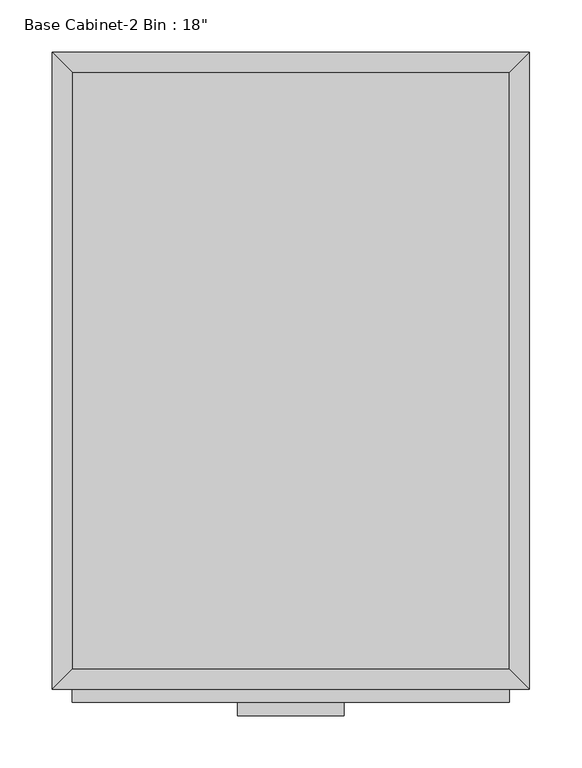
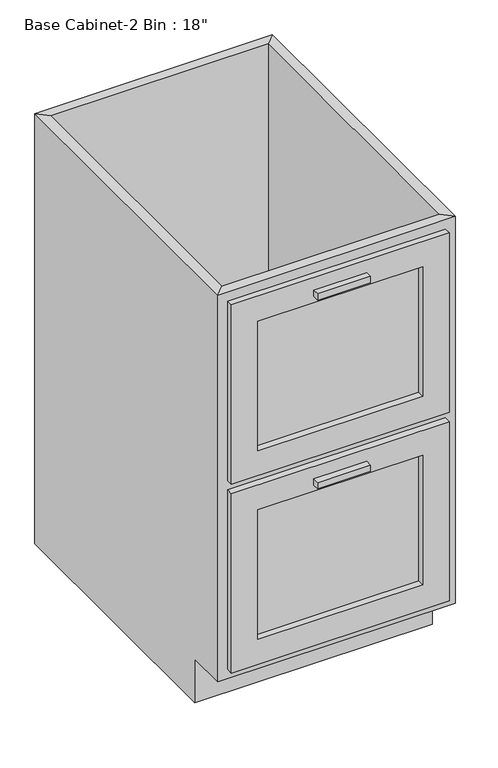
"""IFC4 building model written with IfcOpenShell, lengths in millimetres: furniture geometry."""

from ifc_helpers import new_model, si_unit, frame, origin, place, context, project, spatial, polyline, outline, extrude, faceted_brep, source, transform, mapped, element, save


def furniture_3e5ce493(model_context):
    return source(origin(), model_context, "Body", "SolidModel", [
        extrude(outline(polyline([(69.5377049, -635.0), (-32.0622951, -635.0), (-32.0622951, -622.3), (69.5377049, -622.3), (69.5377049, -635.0)])), frame((0.0, 0.0, 819.15), z_axis=(0.0, 0.0, 1.0), x_axis=(1.0, 0.0, 0.0)), (0.0, 0.0, 1.0), 12.7),
        extrude(outline(polyline([(69.5377049, -635.0), (-32.0622951, -635.0), (-32.0622951, -622.3), (69.5377049, -622.3), (69.5377049, -635.0)])), frame((0.0, 0.0, 434.975), z_axis=(0.0, 0.0, 1.0), x_axis=(1.0, 0.0, 0.0)), (0.0, 0.0, 1.0), 12.7),
        extrude(outline(polyline([(857.25, 228.2877049), (857.25, -190.8122951), (492.125, -190.8122951), (492.125, 228.2877049), (857.25, 228.2877049)]), holes=[polyline([(806.45, 177.4877049), (542.925, 177.4877049), (542.925, -140.0122951), (806.45, -140.0122951), (806.45, 177.4877049)])]), frame((0.0, -622.3, 0.0), z_axis=(0.0, 1.0, 0.0), x_axis=(0.0, 0.0, 1.0)), (0.0, 0.0, 1.0), 12.7),
        extrude(outline(polyline([(473.075, 228.2877049), (473.075, -190.8122951), (107.95, -190.8122951), (107.95, 228.2877049), (473.075, 228.2877049)]), holes=[polyline([(422.275, 177.4877049), (158.75, 177.4877049), (158.75, -140.0122951), (422.275, -140.0122951), (422.275, 177.4877049)])]), frame((0.0, -622.3, 0.0), z_axis=(0.0, 1.0, 0.0), x_axis=(0.0, 0.0, 1.0)), (0.0, 0.0, 1.0), 12.7),
        extrude(outline(polyline([(177.4877049, -609.6), (-140.0122951, -609.6), (-140.0122951, -590.55), (177.4877049, -590.55), (177.4877049, -609.6)])), frame((0.0, 0.0, 542.925), z_axis=(0.0, 0.0, 1.0), x_axis=(1.0, 0.0, 0.0)), (0.0, 0.0, 1.0), 263.525),
        extrude(outline(polyline([(177.4877049, -609.6), (-140.0122951, -609.6), (-140.0122951, -590.55), (177.4877049, -590.55), (177.4877049, -609.6)])), frame((0.0, 0.0, 158.75), z_axis=(0.0, 0.0, 1.0), x_axis=(1.0, 0.0, 0.0)), (0.0, 0.0, 1.0), 263.525),
        extrude(outline(polyline([(228.2877049, -19.05), (228.2877049, -590.55), (-190.8122951, -590.55), (-190.8122951, -19.05), (228.2877049, -19.05)])), frame((0.0, 0.0, 88.9), z_axis=(0.0, 0.0, 1.0), x_axis=(1.0, 0.0, 0.0)), (0.0, 0.0, 1.0), 19.05),
        faceted_brep([(228.2877049, -590.55, 876.3), (228.2877049, -590.55, 88.9), (-190.8122951, -590.55, 88.9), (-190.8122951, -590.55, 876.3), (177.4877049, -590.55, 542.925), (177.4877049, -590.55, 806.45), (-140.0122951, -590.55, 806.45), (-140.0122951, -590.55, 542.925), (177.4877049, -590.55, 158.75), (177.4877049, -590.55, 422.275), (-140.0122951, -590.55, 422.275), (-140.0122951, -590.55, 158.75), (-209.8622951, -609.6, 876.3), (247.3377049, -609.6, 876.3), (-209.8622951, -609.6, 88.9), (247.3377049, -609.6, 88.9), (177.4877049, -609.6, 806.45), (177.4877049, -609.6, 542.925), (-140.0122951, -609.6, 542.925), (-140.0122951, -609.6, 806.45), (177.4877049, -609.6, 422.275), (177.4877049, -609.6, 158.75), (-140.0122951, -609.6, 158.75), (-140.0122951, -609.6, 422.275), (-190.8122951, -533.4, 88.9), (-190.8122951, -19.05, 88.9), (-190.8122951, -19.05, 876.3), (-209.8622951, 0.0, 876.3), (-209.8622951, 0.0, 0.0), (-209.8622951, -533.4, 0.0), (-209.8622951, -533.4, 88.9), (228.2877049, -19.05, 88.9), (228.2877049, -19.05, 876.3), (247.3377049, 0.0, 876.3), (247.3377049, 0.0, 0.0), (228.2877049, -533.4, 88.9), (247.3377049, -533.4, 88.9), (247.3377049, -533.4, 0.0)], [[[0, 1, 2, 3], [4, 5, 6, 7], [8, 9, 10, 11]], [[0, 3, 12, 13]], [[13, 12, 14, 15], [16, 17, 18, 19], [20, 21, 22, 23]], [[2, 1, 15, 14]], [[3, 2, 24, 25, 26]], [[12, 3, 26, 27]], [[14, 12, 27, 28, 29, 30]], [[2, 14, 30, 24]], [[26, 25, 31, 32]], [[27, 26, 32, 33]], [[27, 33, 34, 28]], [[1, 0, 32, 31, 35]], [[0, 13, 33, 32]], [[13, 15, 36, 37, 34, 33]], [[15, 1, 35, 36]], [[24, 35, 31, 25]], [[34, 37, 29, 28]], [[29, 37, 36, 35, 24, 30]], [[4, 17, 16, 5]], [[17, 4, 7, 18]], [[18, 7, 6, 19]], [[5, 16, 19, 6]], [[8, 21, 20, 9]], [[21, 8, 11, 22]], [[22, 11, 10, 23]], [[9, 20, 23, 10]]]),
    ])


if __name__ == "__main__":
    model = new_model("IFC4")
    model_context = context("Model", 3, world=origin())
    ifc_project = project(units=[si_unit("LENGTHUNIT", "METRE", prefix="MILLI")], contexts=[model_context])
    site = spatial("IfcSite", under=ifc_project)
    building = spatial("IfcBuilding", under=site)
    placement = place(None, origin())
    furniture_shape = furniture_3e5ce493(model_context)
    element("IfcFurniture", 1, ObjectType="Base Cabinet-2 Bin : 18\"", at=placement, inside=building, context=model_context, shape_type="MappedRepresentation", body=[
        mapped(furniture_shape, transform((0.0, 0.0, 0.0), x_axis=(1.0, 0.0, 0.0), y_axis=(0.0, 1.0, 0.0), z_axis=(0.0, 0.0, 1.0))),
    ])
    save(model, "model.ifc")

# Revit data of these elements
# Type "Base Cabinet-2 Bin : 18\""
#   Assembly Code = "C1030410"
#   Depth = 2' - 0"
#   Height = 2' - 10 1/2"
#   Toe Depth = 0' - 3"
#   Toe Height = 0' - 3 1/2"
#   Width = 1' - 6"
#   Cabinet Material = none
#   Door/Drawer Material = none
#   Handle Material = Cabinets - Handles
#   Panels = none
#   Default Elevation = 0
# Element 1 (IfcFurniture, "Base Cabinet-2 Bin : 18\"")
#   Materials on its faces: "Cabinets", "Cabinets - Handles", "Cabinets - Panel/Glass"
# Materials
#   "Cabinets - Handles": class "Metal", colour RGB 57 57 57, transparency 0
#   "Cabinets": colour RGB 249 249 249, transparency 0
#   "Cabinets - Panel/Glass": colour RGB 252 255 255, transparency 0.72
